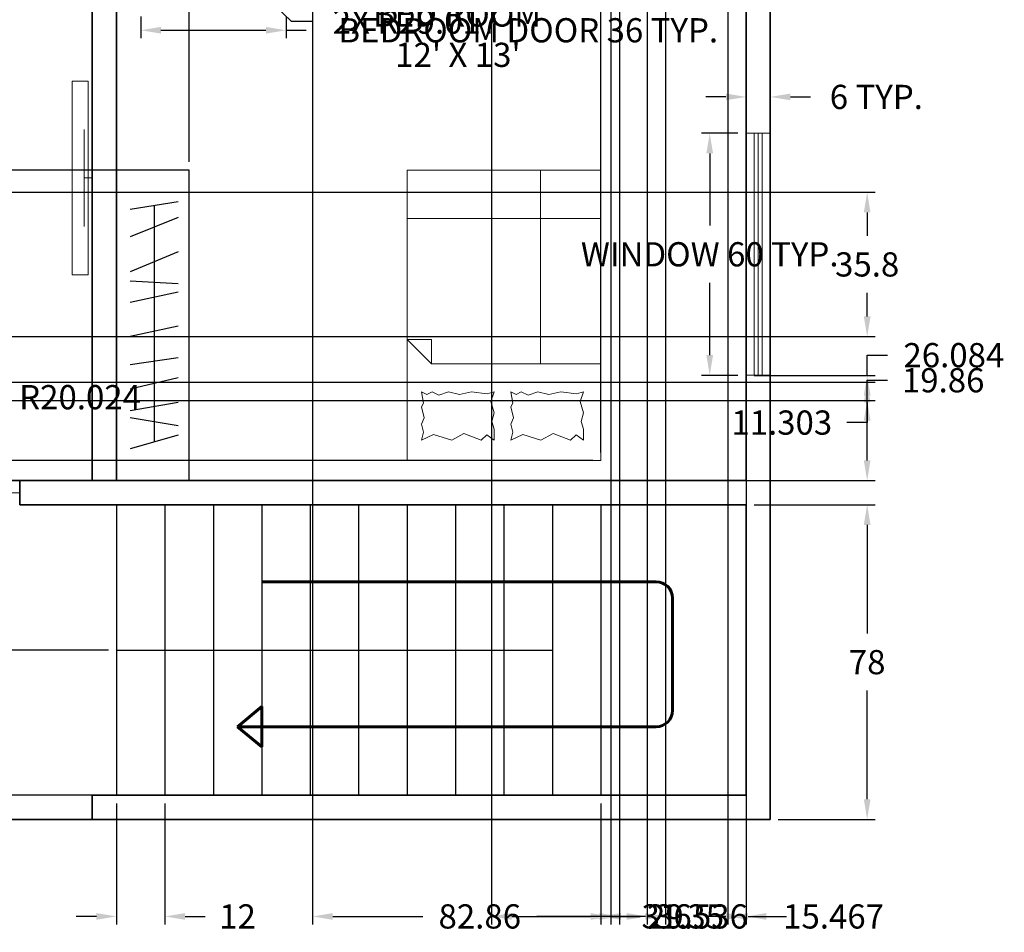
# Model space of a CAD drawing. Units: inches. Extents: x 185 to 668, y 153 to 689.
# Tile 2 of 5: x 417 to 661, y 153 to 380. Entities that reach past the tile are written whole.
import ezdxf

# ---------------------------------------------------------------- set-up
doc = ezdxf.new("R2010")
doc.units = ezdxf.units.IN
doc.header["$MEASUREMENT"] = 0
for name, color, linetype, lineweight in [('A-ANNO-DIMS', 2, 'Continuous', 18), ('A-ANNO-SYMB', 2, 'Continuous', 60), ('A-AREA-IDEN', 7, 'Continuous', 25), ('A-DOOR', 3, 'Continuous', 18), ('A-EQPM', 9, 'Continuous', 18), ('A-FLOR-CASE', 8, 'Continuous', 25), ('A-FLOR-STRS', 7, 'Continuous', 25), ('A-FURN', 8, 'Continuous', 18), ('A-GLAZ', 4, 'Continuous', 18), ('A-WALL', 7, 'Continuous', 35)]:
    doc.layers.add(name, color=color, linetype=linetype, lineweight=lineweight)
doc.styles.get("Standard").update_dxf_attribs({"font": 'arial.ttf'})
doc.dimstyles.get("Standard").update_dxf_attribs({"dimtxt": 6, "dimasz": 5, "dimexe": 2, "dimexo": 2, "dimgap": 4, "dimtad": 0, "dimtih": 1, "dimtoh": 1, "dimdec": 0, "dimzin": 0, "dimdsep": 46, "dimlunit": 3, "dimtxsty": 'Standard', "dimcen": 2, "dimadec": 0, "dimazin": 0, "dimtfac": 1, "dimtdec": 0, "dimtofl": 0, "dimtmove": 0, "dimatfit": 3, "dimfxl": 1, "dimtolj": 1, "dimtzin": 0, "dimarcsym": 0})

# ---------------------------------------------------------------- blocks, each defined once
blk = doc.blocks.new('BED-DOUBLE-48X72')
for p, q in [((0, 72), (48, 72)), ((0, 0), (0, 72)), ((0, 72), (48, 72)), ((0, 0), (0, 72)), ((48, 72), (48, 0)), ((3.52, 66.93), (6.5, 65.56)), ((4.06, 65), (3.52, 66.93)), ((3.52, 66.93), (6.5, 65.56)), ((4.06, 65), (3.52, 66.93)), ((6.5, 65.56), (11.02, 66.93)), ((6.5, 65.56), (11.02, 66.93)), ((11.02, 66.93), (14.02, 65.28)), ((11.02, 66.93), (14.02, 65.28)), ((14.02, 65.28), (18.3, 66.93)), ((14.02, 65.28), (18.3, 66.93)), ((18.3, 66.93), (19.74, 65.6)), ((18.3, 66.93), (19.74, 65.6)), ((19.74, 65.6), (21.52, 66.93)), ((19.74, 65.6), (21.52, 66.93)), ((21.52, 66.93), (21.52, 64.24)), ((21.52, 66.93), (21.52, 64.24)), ((25.65, 66.93), (28.63, 65.56)), ((26.19, 65), (25.65, 66.93)), ((25.65, 66.93), (28.63, 65.56)), ((26.19, 65), (25.65, 66.93)), ((28.63, 65.56), (33.15, 66.93)), ((28.63, 65.56), (33.15, 66.93)), ((33.15, 66.93), (36.15, 65.28)), ((33.15, 66.93), (36.15, 65.28)), ((36.15, 65.28), (40.43, 66.93)), ((36.15, 65.28), (40.43, 66.93)), ((40.43, 66.93), (41.87, 65.6)), ((40.43, 66.93), (41.87, 65.6)), ((41.87, 65.6), (43.65, 66.93)), ((41.87, 65.6), (43.65, 66.93)), ((43.65, 66.93), (43.65, 64.24)), ((43.65, 66.93), (43.65, 64.24)), ((3.52, 63), (4.06, 65)), ((3.52, 63), (4.06, 65)), ((21.52, 64.24), (20.98, 62.32)), ((21.52, 64.24), (20.98, 62.32)), ((25.65, 63), (26.19, 65)), ((25.65, 63), (26.19, 65)), ((43.65, 64.24), (43.11, 62.32)), ((43.65, 64.24), (43.11, 62.32)), ((4.22, 61.4), (3.52, 63)), ((4.22, 61.4), (3.52, 63)), ((3.52, 58.72), (4.22, 61.4)), ((3.52, 58.72), (4.22, 61.4)), ((20.98, 62.32), (21.52, 60.2)), ((20.98, 62.32), (21.52, 60.2)), ((26.35, 61.4), (25.65, 63)), ((26.35, 61.4), (25.65, 63)), ((25.65, 58.72), (26.35, 61.4)), ((25.65, 58.72), (26.35, 61.4)), ((43.11, 62.32), (43.65, 60.2)), ((43.11, 62.32), (43.65, 60.2)), ((4.06, 57.76), (3.52, 58.72)), ((4.06, 57.76), (3.52, 58.72)), ((21.52, 60.2), (20.7, 57.36)), ((21.52, 60.2), (20.7, 57.36)), ((26.19, 57.76), (25.65, 58.72)), ((26.19, 57.76), (25.65, 58.72)), ((43.65, 60.2), (42.83, 57.36)), ((43.65, 60.2), (42.83, 57.36)), ((3.52, 54.93), (4.06, 57.76)), ((3.52, 54.93), (4.06, 57.76)), ((20.7, 57.36), (21.52, 54.93)), ((20.7, 57.36), (21.52, 54.93)), ((25.65, 54.93), (26.19, 57.76)), ((25.65, 54.93), (26.19, 57.76)), ((42.83, 57.36), (43.65, 54.93)), ((42.83, 57.36), (43.65, 54.93)), ((4.9, 55.65), (3.52, 54.93)), ((4.9, 55.65), (3.52, 54.93)), ((6.14, 54.93), (4.9, 55.65)), ((6.14, 54.93), (4.9, 55.65)), ((7.86, 55.8), (6.14, 54.93)), ((7.86, 55.8), (6.14, 54.93)), ((10.22, 54.93), (7.86, 55.8)), ((10.22, 54.93), (7.86, 55.8)), ((12.98, 55.61), (10.22, 54.93)), ((12.98, 55.61), (10.22, 54.93)), ((15.94, 54.93), (12.98, 55.61)), ((15.94, 54.93), (12.98, 55.61)), ((19.78, 55.49), (15.94, 54.93)), ((19.78, 55.49), (15.94, 54.93)), ((21.52, 54.93), (19.78, 55.49)), ((21.52, 54.93), (19.78, 55.49)), ((27.03, 55.65), (25.65, 54.93)), ((27.03, 55.65), (25.65, 54.93)), ((28.27, 54.93), (27.03, 55.65)), ((28.27, 54.93), (27.03, 55.65)), ((29.99, 55.8), (28.27, 54.93)), ((29.99, 55.8), (28.27, 54.93)), ((32.35, 54.93), (29.99, 55.8)), ((32.35, 54.93), (29.99, 55.8)), ((35.11, 55.61), (32.35, 54.93)), ((35.11, 55.61), (32.35, 54.93)), ((38.07, 54.93), (35.11, 55.61)), ((38.07, 54.93), (35.11, 55.61)), ((41.91, 55.49), (38.07, 54.93)), ((41.91, 55.49), (38.07, 54.93)), ((43.65, 54.93), (41.91, 55.49)), ((43.65, 54.93), (41.91, 55.49)), ((0, 42), (6, 48)), ((0, 42), (6, 48)), ((6, 48), (48, 48)), ((6, 48), (6, 42)), ((6, 48), (48, 48)), ((6, 48), (6, 42)), ((33, 48), (33, 0)), ((33, 48), (33, 0)), ((0, 42), (0, 0)), ((0, 42), (6, 42)), ((0, 42), (0, 0)), ((0, 42), (6, 42)), ((48, 12), (0, 12)), ((48, 12), (0, 12)), ((48, 0), (0, 0)), ((48, 0), (0, 0))]:
    blk.add_line(p, q)
blk = doc.blocks.new('WINDOW-60')
for p, q in [((2, 60), (0, 60)), ((2, 60), (2, 0)), ((4, 60), (2, 60)), ((3, 0), (3, 60)), ((4, 0), (4, 60)), ((4, 60), (6, 60)), ((6, 0), (0, 0)), ((2, 0), (0, 0)), ((2, 0), (4, 0)), ((4, 0), (6, 0))]:
    blk.add_line(p, q)
blk = doc.blocks.new('*D9')
at = {"layer": 'A-ANNO-DIMS', "color": 0, "lineweight": -2, "transparency": 16777216}
for p, q in [((595.04, 351.46), (586.04, 351.46)), ((588.04, 346.46), (588.04, 328.57)), ((588.04, 296.46), (588.04, 314.36)), ((595.04, 291.46), (586.04, 291.46))]:
    blk.add_line(p, q, dxfattribs=at)
at = {"layer": 'A-ANNO-DIMS', "color": 0, "transparency": 16777216}
for points in [[(587.21, 346.46), (588.87, 346.46), (588.04, 351.46)], [(587.21, 296.46), (588.87, 296.46), (588.04, 291.46)]]:
    blk.add_solid(points, dxfattribs=at)
at = {"layer": 'Defpoints', "color": 0, "transparency": 16777216}
for p in [(588.04, 351.46), (597.04, 351.46), (597.04, 291.46)]:
    blk.add_point(p, dxfattribs=at)
at = {"layer": 'A-ANNO-DIMS', "color": 0, "transparency": 16777216, "insert": (588.04, 321.46), "char_height": 6, "attachment_point": 5}
blk.add_mtext('\\A1;WINDOW 60 TYP.', dxfattribs=at)
blk = doc.blocks.new('*D10')
at = {"layer": 'A-ANNO-DIMS', "color": 0, "lineweight": -2, "transparency": 16777216}
for p, q in [((597.04, 353.46), (597.04, 362.46)), ((603.04, 353.46), (603.04, 362.46)), ((592.04, 360.46), (587.04, 360.46)), ((608.04, 360.46), (613.04, 360.46))]:
    blk.add_line(p, q, dxfattribs=at)
at = {"layer": 'A-ANNO-DIMS', "color": 0, "transparency": 16777216}
for points in [[(592.04, 361.3), (592.04, 359.63), (597.04, 360.46)], [(608.04, 361.3), (608.04, 359.63), (603.04, 360.46)]]:
    blk.add_solid(points, dxfattribs=at)
at = {"layer": 'Defpoints', "color": 0, "transparency": 16777216}
for p in [(603.04, 360.46), (597.04, 351.46), (603.04, 351.46)]:
    blk.add_point(p, dxfattribs=at)
at = {"layer": 'A-ANNO-DIMS', "color": 0, "transparency": 16777216, "insert": (629.33, 360.46), "char_height": 6, "attachment_point": 5}
blk.add_mtext('\\A1;6 TYP.', dxfattribs=at)
blk = doc.blocks.new('*D21')
at = {"layer": 'A-ANNO-DIMS', "color": 0, "lineweight": -2, "transparency": 16777216}
for p, q in [((447.04, 380.38), (447.04, 374.98)), ((483.04, 380.38), (483.04, 374.98)), ((452.04, 376.98), (478.04, 376.98)), ((483.04, 376.98), (488.04, 376.98))]:
    blk.add_line(p, q, dxfattribs=at)
at = {"layer": 'A-ANNO-DIMS', "color": 0, "transparency": 16777216}
for points in [[(452.04, 377.81), (452.04, 376.15), (447.04, 376.98)], [(478.04, 377.81), (478.04, 376.15), (483.04, 376.98)]]:
    blk.add_solid(points, dxfattribs=at)
at = {"layer": 'Defpoints', "color": 0, "transparency": 16777216}
for p in [(447.04, 382.38), (483.04, 382.38), (483.04, 376.98)]:
    blk.add_point(p, dxfattribs=at)
at = {"layer": 'A-ANNO-DIMS', "color": 0, "transparency": 16777216, "insert": (543.07, 376.98), "char_height": 6, "attachment_point": 5}
blk.add_mtext('\\A1;BEDROOM DOOR 36 TYP.', dxfattribs=at)
blk = doc.blocks.new('*D27')
at = {"layer": 'A-ANNO-DIMS', "color": 0, "lineweight": -2, "transparency": 16777216}
for p, q in [((599.04, 259.38), (629.06, 259.38)), ((627.06, 254.38), (627.06, 227.44)), ((627.06, 186.38), (627.06, 213.32)), ((605.04, 181.38), (629.06, 181.38))]:
    blk.add_line(p, q, dxfattribs=at)
at = {"layer": 'A-ANNO-DIMS', "color": 0, "transparency": 16777216}
for points in [[(626.23, 254.38), (627.89, 254.38), (627.06, 259.38)], [(626.23, 186.38), (627.89, 186.38), (627.06, 181.38)]]:
    blk.add_solid(points, dxfattribs=at)
at = {"layer": 'Defpoints', "color": 0, "transparency": 16777216}
for p in [(597.04, 259.38), (627.06, 259.38), (603.04, 181.38)]:
    blk.add_point(p, dxfattribs=at)
at = {"layer": 'A-ANNO-DIMS', "color": 0, "transparency": 16777216, "insert": (627.06, 220.38), "char_height": 6, "attachment_point": 5}
blk.add_mtext('\\A1;78', dxfattribs=at)
blk = doc.blocks.new('*D28')
at = {"layer": 'A-ANNO-DIMS', "color": 0, "lineweight": -2, "transparency": 16777216}
for p, q in [((627.06, 285.24), (627.06, 290.24)), ((627.06, 290.24), (632.06, 290.24)), ((251.04, 285.24), (629.06, 285.24)), ((627.06, 270.38), (627.06, 280.24)), ((251.04, 265.38), (629.06, 265.38))]:
    blk.add_line(p, q, dxfattribs=at)
at = {"layer": 'A-ANNO-DIMS', "color": 0, "transparency": 16777216}
for points in [[(626.23, 280.24), (627.89, 280.24), (627.06, 285.24)], [(626.23, 270.38), (627.89, 270.38), (627.06, 265.38)]]:
    blk.add_solid(points, dxfattribs=at)
at = {"layer": 'Defpoints', "color": 0, "transparency": 16777216}
for p in [(249.04, 285.24), (627.06, 285.24), (249.04, 265.38)]:
    blk.add_point(p, dxfattribs=at)
at = {"layer": 'A-ANNO-DIMS', "color": 0, "transparency": 16777216, "insert": (645.9, 290.24), "char_height": 6, "attachment_point": 5}
blk.add_mtext('\\A1;19.86', dxfattribs=at)
blk = doc.blocks.new('*D29')
at = {"layer": 'A-ANNO-DIMS', "color": 0, "lineweight": -2, "transparency": 16777216}
for p, q in [((627.06, 291.46), (627.06, 296.46)), ((627.06, 296.46), (632.06, 296.46)), ((599.04, 291.46), (629.06, 291.46)), ((627.06, 270.38), (627.06, 286.46)), ((599.04, 265.38), (629.06, 265.38))]:
    blk.add_line(p, q, dxfattribs=at)
at = {"layer": 'A-ANNO-DIMS', "color": 0, "transparency": 16777216}
for points in [[(626.23, 286.46), (627.89, 286.46), (627.06, 291.46)], [(626.23, 270.38), (627.89, 270.38), (627.06, 265.38)]]:
    blk.add_solid(points, dxfattribs=at)
at = {"layer": 'Defpoints', "color": 0, "transparency": 16777216}
for p in [(597.04, 291.46), (627.06, 291.46), (597.04, 265.38)]:
    blk.add_point(p, dxfattribs=at)
at = {"layer": 'A-ANNO-DIMS', "color": 0, "transparency": 16777216, "insert": (648.55, 296.46), "char_height": 6, "attachment_point": 5}
blk.add_mtext('\\A1;26.084', dxfattribs=at)
blk = doc.blocks.new('*D33')
at = {"layer": 'A-ANNO-DIMS', "color": 0, "lineweight": -2, "transparency": 16777216}
for p, q in [((565.69, 653.38), (565.69, 155.36)), ((597.04, 653.38), (597.04, 155.36)), ((560.69, 157.36), (555.69, 157.36)), ((602.04, 157.36), (607.04, 157.36))]:
    blk.add_line(p, q, dxfattribs=at)
at = {"layer": 'A-ANNO-DIMS', "color": 0, "transparency": 16777216}
for points in [[(560.69, 158.19), (560.69, 156.53), (565.69, 157.36)], [(602.04, 158.19), (602.04, 156.53), (597.04, 157.36)]]:
    blk.add_solid(points, dxfattribs=at)
at = {"layer": 'Defpoints', "color": 0, "transparency": 16777216}
for p in [(565.69, 655.38), (597.04, 655.38), (597.04, 157.36)]:
    blk.add_point(p, dxfattribs=at)
at = {"layer": 'A-ANNO-DIMS', "color": 0, "transparency": 16777216, "insert": (581.37, 157.36), "char_height": 6, "attachment_point": 5}
blk.add_mtext('\\A1;31.35', dxfattribs=at)
blk = doc.blocks.new('*D39')
at = {"layer": 'A-ANNO-DIMS', "color": 0, "lineweight": -2, "transparency": 16777216}
for p, q in [((441.04, 185.38), (441.04, 155.36)), ((453.04, 185.38), (453.04, 155.36)), ((436.04, 157.36), (431.04, 157.36)), ((458.04, 157.36), (463.04, 157.36))]:
    blk.add_line(p, q, dxfattribs=at)
at = {"layer": 'A-ANNO-DIMS', "color": 0, "transparency": 16777216}
for points in [[(436.04, 158.19), (436.04, 156.53), (441.04, 157.36)], [(458.04, 158.19), (458.04, 156.53), (453.04, 157.36)]]:
    blk.add_solid(points, dxfattribs=at)
at = {"layer": 'Defpoints', "color": 0, "transparency": 16777216}
for p in [(441.04, 187.38), (453.04, 187.38), (453.04, 157.36)]:
    blk.add_point(p, dxfattribs=at)
at = {"layer": 'A-ANNO-DIMS', "color": 0, "transparency": 16777216, "insert": (471.03, 157.36), "char_height": 6, "attachment_point": 5}
blk.add_mtext('\\A1;12', dxfattribs=at)
blk = doc.blocks.new('*D43')
at = {"layer": 'A-ANNO-DIMS', "color": 0, "lineweight": -2, "transparency": 16777216}
for p, q in [((489.63, 629.38), (489.63, 155.36)), ((572.5, 629.38), (572.5, 155.36)), ((494.63, 157.36), (516.94, 157.36)), ((567.5, 157.36), (545.19, 157.36))]:
    blk.add_line(p, q, dxfattribs=at)
at = {"layer": 'A-ANNO-DIMS', "color": 0, "transparency": 16777216}
for points in [[(494.63, 158.19), (494.63, 156.53), (489.63, 157.36)], [(567.5, 158.19), (567.5, 156.53), (572.5, 157.36)]]:
    blk.add_solid(points, dxfattribs=at)
at = {"layer": 'Defpoints', "color": 0, "transparency": 16777216}
for p in [(489.63, 631.38), (572.5, 631.38), (572.5, 157.36)]:
    blk.add_point(p, dxfattribs=at)
at = {"layer": 'A-ANNO-DIMS', "color": 0, "transparency": 16777216, "insert": (531.06, 157.36), "char_height": 6, "attachment_point": 5}
blk.add_mtext('\\A1;82.86', dxfattribs=at)
blk = doc.blocks.new('*D52')
at = {"layer": 'A-ANNO-DIMS', "color": 0, "lineweight": -2, "transparency": 16777216}
for p, q in [((441.04, 344.34), (441.04, 687.4)), ((459.04, 344.34), (459.04, 687.4)), ((436.04, 685.4), (431.04, 685.4)), ((464.04, 685.4), (469.04, 685.4))]:
    blk.add_line(p, q, dxfattribs=at)
at = {"layer": 'A-ANNO-DIMS', "color": 0, "transparency": 16777216}
for points in [[(436.04, 686.23), (436.04, 684.56), (441.04, 685.4)], [(464.04, 686.23), (464.04, 684.56), (459.04, 685.4)]]:
    blk.add_solid(points, dxfattribs=at)
at = {"layer": 'Defpoints', "color": 0, "transparency": 16777216}
for p in [(459.04, 685.4), (441.04, 342.34), (459.04, 342.34)]:
    blk.add_point(p, dxfattribs=at)
at = {"layer": 'A-ANNO-DIMS', "color": 0, "transparency": 16777216, "insert": (450.04, 685.4), "char_height": 6, "attachment_point": 5}
blk.add_mtext('\\A1;18', dxfattribs=at)
blk = doc.blocks.new('*D53')
at = {"layer": 'A-ANNO-DIMS', "color": 0, "lineweight": -2, "transparency": 16777216}
for p, q in [((457.04, 342.34), (217.02, 342.34)), ((219.02, 337.34), (219.02, 310.92)), ((219.02, 270.38), (219.02, 296.79)), ((457.04, 265.38), (217.02, 265.38))]:
    blk.add_line(p, q, dxfattribs=at)
at = {"layer": 'A-ANNO-DIMS', "color": 0, "transparency": 16777216}
for points in [[(218.19, 337.34), (219.86, 337.34), (219.02, 342.34)], [(218.19, 270.38), (219.86, 270.38), (219.02, 265.38)]]:
    blk.add_solid(points, dxfattribs=at)
at = {"layer": 'Defpoints', "color": 0, "transparency": 16777216}
for p in [(219.02, 342.34), (459.04, 342.34), (459.04, 265.38)]:
    blk.add_point(p, dxfattribs=at)
at = {"layer": 'A-ANNO-DIMS', "color": 0, "transparency": 16777216, "insert": (219.02, 303.86), "char_height": 6, "attachment_point": 5}
blk.add_mtext('\\A1;76.96', dxfattribs=at)
blk = doc.blocks.new('*D55')
at = {"layer": 'A-ANNO-DIMS', "color": 0, "lineweight": -2, "transparency": 16777216}
for p, q in [((313.16, 336.85), (629.06, 336.85)), ((627.06, 331.85), (627.06, 326.02)), ((627.06, 306.05), (627.06, 311.89)), ((313.16, 301.05), (629.06, 301.05))]:
    blk.add_line(p, q, dxfattribs=at)
at = {"layer": 'A-ANNO-DIMS', "color": 0, "transparency": 16777216}
for points in [[(626.23, 331.85), (627.89, 331.85), (627.06, 336.85)], [(626.23, 306.05), (627.89, 306.05), (627.06, 301.05)]]:
    blk.add_solid(points, dxfattribs=at)
at = {"layer": 'Defpoints', "color": 0, "transparency": 16777216}
for p in [(311.16, 336.85), (627.06, 336.85), (311.16, 301.05)]:
    blk.add_point(p, dxfattribs=at)
at = {"layer": 'A-ANNO-DIMS', "color": 0, "transparency": 16777216, "insert": (627.06, 318.95), "char_height": 6, "attachment_point": 5}
blk.add_mtext('\\A1;35.8', dxfattribs=at)
blk = doc.blocks.new('*D59')
at = {"layer": 'A-ANNO-DIMS', "color": 0, "lineweight": -2, "transparency": 16777216}
for p, q in [((627.06, 306.05), (627.06, 311.05)), ((289.14, 301.05), (629.06, 301.05)), ((297.85, 289.75), (629.06, 289.75)), ((627.06, 284.75), (627.06, 279.75)), ((627.06, 279.75), (622.06, 279.75))]:
    blk.add_line(p, q, dxfattribs=at)
at = {"layer": 'A-ANNO-DIMS', "color": 0, "transparency": 16777216}
for points in [[(626.23, 306.05), (627.89, 306.05), (627.06, 301.05)], [(626.23, 284.75), (627.89, 284.75), (627.06, 289.75)]]:
    blk.add_solid(points, dxfattribs=at)
at = {"layer": 'Defpoints', "color": 0, "transparency": 16777216}
for p in [(287.14, 301.05), (295.85, 289.75), (627.06, 289.75)]:
    blk.add_point(p, dxfattribs=at)
at = {"layer": 'A-ANNO-DIMS', "color": 0, "transparency": 16777216, "insert": (605.89, 279.75), "char_height": 6, "attachment_point": 5}
blk.add_mtext('\\A1;11.303', dxfattribs=at)
blk = doc.blocks.new('*D60')
at = {"layer": 'A-ANNO-DIMS', "color": 0, "lineweight": -2, "transparency": 16777216}
for p, q in [((439.04, 223.38), (217.02, 223.38)), ((219.02, 218.38), (219.02, 212.44)), ((219.02, 192.38), (219.02, 198.31)), ((439.04, 187.38), (217.02, 187.38))]:
    blk.add_line(p, q, dxfattribs=at)
at = {"layer": 'A-ANNO-DIMS', "color": 0, "transparency": 16777216}
for points in [[(218.19, 218.38), (219.86, 218.38), (219.02, 223.38)], [(218.19, 192.38), (219.86, 192.38), (219.02, 187.38)]]:
    blk.add_solid(points, dxfattribs=at)
at = {"layer": 'Defpoints', "color": 0, "transparency": 16777216}
for p in [(219.02, 223.38), (441.04, 223.38), (441.04, 187.38)]:
    blk.add_point(p, dxfattribs=at)
at = {"layer": 'A-ANNO-DIMS', "color": 0, "transparency": 16777216, "insert": (219.02, 205.38), "char_height": 6, "attachment_point": 5}
blk.add_mtext('\\A1;36', dxfattribs=at)
blk = doc.blocks.new('*D61')
at = {"layer": 'A-ANNO-DIMS', "color": 0, "lineweight": -2, "transparency": 16777216}
for p, q in [((561.04, 185.38), (561.04, 155.36)), ((597.04, 185.38), (597.04, 155.36)), ((566.04, 157.36), (570.75, 157.36)), ((592.04, 157.36), (587.33, 157.36))]:
    blk.add_line(p, q, dxfattribs=at)
at = {"layer": 'A-ANNO-DIMS', "color": 0, "transparency": 16777216}
for points in [[(566.04, 158.19), (566.04, 156.53), (561.04, 157.36)], [(592.04, 158.19), (592.04, 156.53), (597.04, 157.36)]]:
    blk.add_solid(points, dxfattribs=at)
at = {"layer": 'Defpoints', "color": 0, "transparency": 16777216}
for p in [(561.04, 187.38), (597.04, 187.38), (597.04, 157.36)]:
    blk.add_point(p, dxfattribs=at)
at = {"layer": 'A-ANNO-DIMS', "color": 0, "transparency": 16777216, "insert": (579.04, 157.36), "char_height": 6, "attachment_point": 5}
blk.add_mtext('\\A1;36', dxfattribs=at)
blk = doc.blocks.new('*D62')
at = {"layer": 'A-ANNO-DIMS', "color": 0, "lineweight": -2, "transparency": 16777216}
for p, q in [((533.97, 632.47), (533.97, 155.36)), ((563.51, 632.47), (563.51, 155.36)), ((538.97, 157.36), (558.51, 157.36)), ((563.51, 157.36), (568.51, 157.36))]:
    blk.add_line(p, q, dxfattribs=at)
at = {"layer": 'A-ANNO-DIMS', "color": 0, "transparency": 16777216}
for points in [[(538.97, 158.19), (538.97, 156.53), (533.97, 157.36)], [(558.51, 158.19), (558.51, 156.53), (563.51, 157.36)]]:
    blk.add_solid(points, dxfattribs=at)
at = {"layer": 'Defpoints', "color": 0, "transparency": 16777216}
for p in [(533.97, 634.47), (563.51, 634.47), (563.51, 157.36)]:
    blk.add_point(p, dxfattribs=at)
at = {"layer": 'A-ANNO-DIMS', "color": 0, "transparency": 16777216, "insert": (585.01, 157.36), "char_height": 6, "attachment_point": 5}
blk.add_mtext('\\A1;29.536', dxfattribs=at)
blk = doc.blocks.new('*D65')
at = {"layer": 'A-ANNO-DIMS', "color": 0, "lineweight": -2, "transparency": 16777216}
for p, q in [((577.09, 545.77), (577.09, 155.36)), ((592.55, 545.77), (592.55, 155.36)), ((572.09, 157.36), (567.09, 157.36)), ((597.55, 157.36), (602.55, 157.36))]:
    blk.add_line(p, q, dxfattribs=at)
at = {"layer": 'A-ANNO-DIMS', "color": 0, "transparency": 16777216}
for points in [[(572.09, 158.19), (572.09, 156.53), (577.09, 157.36)], [(597.55, 158.19), (597.55, 156.53), (592.55, 157.36)]]:
    blk.add_solid(points, dxfattribs=at)
at = {"layer": 'Defpoints', "color": 0, "transparency": 16777216}
for p in [(577.09, 547.77), (592.55, 547.77), (592.55, 157.36)]:
    blk.add_point(p, dxfattribs=at)
at = {"layer": 'A-ANNO-DIMS', "color": 0, "transparency": 16777216, "insert": (618.73, 157.36), "char_height": 6, "attachment_point": 5}
blk.add_mtext('\\A1;15.467', dxfattribs=at)
blk = doc.blocks.new('*D74')
at = {"layer": 'A-ANNO-DIMS', "color": 0, "lineweight": -2, "transparency": 16777216}
for p, q in [((561.08, 272.34), (561.08, 687.4)), ((597.04, 267.38), (597.04, 687.4)), ((556.08, 685.4), (551.08, 685.4)), ((602.04, 685.4), (607.04, 685.4))]:
    blk.add_line(p, q, dxfattribs=at)
at = {"layer": 'A-ANNO-DIMS', "color": 0, "transparency": 16777216}
for points in [[(556.08, 686.23), (556.08, 684.56), (561.08, 685.4)], [(602.04, 686.23), (602.04, 684.56), (597.04, 685.4)]]:
    blk.add_solid(points, dxfattribs=at)
at = {"layer": 'Defpoints', "color": 0, "transparency": 16777216}
for p in [(597.04, 685.4), (561.08, 270.34), (597.04, 265.38)]:
    blk.add_point(p, dxfattribs=at)
at = {"layer": 'A-ANNO-DIMS', "color": 0, "transparency": 16777216, "insert": (579.06, 685.4), "char_height": 6, "attachment_point": 5}
blk.add_mtext('\\A1;35.96', dxfattribs=at)
blk = doc.blocks.new('*D75')
at = {"layer": 'A-ANNO-DIMS', "color": 0, "lineweight": -2, "transparency": 16777216}
for p, q in [((219.02, 275.34), (219.02, 280.34)), ((559.08, 270.34), (217.02, 270.34)), ((595.04, 265.38), (217.02, 265.38)), ((219.02, 260.38), (219.02, 255.38)), ((219.02, 255.38), (214.02, 255.38))]:
    blk.add_line(p, q, dxfattribs=at)
at = {"layer": 'A-ANNO-DIMS', "color": 0, "transparency": 16777216}
for points in [[(218.19, 275.34), (219.86, 275.34), (219.02, 270.34)], [(218.19, 260.38), (219.86, 260.38), (219.02, 265.38)]]:
    blk.add_solid(points, dxfattribs=at)
at = {"layer": 'Defpoints', "color": 0, "transparency": 16777216}
for p in [(561.08, 270.34), (219.02, 265.38), (597.04, 265.38)]:
    blk.add_point(p, dxfattribs=at)
at = {"layer": 'A-ANNO-DIMS', "color": 0, "transparency": 16777216, "insert": (199.78, 255.38), "char_height": 6, "attachment_point": 5}
blk.add_mtext('\\A1;4.957', dxfattribs=at)
blk = doc.blocks.new('*D76')
at = {"layer": 'A-ANNO-DIMS', "color": 0, "lineweight": -2, "transparency": 16777216}
for p, q in [((395.66, 286.05), (390.71, 281.08)), ((400.66, 286.05), (395.66, 286.05)), ((373.04, 261.36), (373.04, 265.36)), ((371.04, 263.36), (375.04, 263.36))]:
    blk.add_line(p, q, dxfattribs=at)
at = {"layer": 'A-ANNO-DIMS', "color": 0, "transparency": 16777216}
blk.add_solid([(390.12, 281.67), (391.3, 280.49), (387.18, 277.54)], dxfattribs=at)
at = {"layer": 'Defpoints', "color": 0, "transparency": 16777216}
for p in [(387.18, 277.54), (373.04, 263.36)]:
    blk.add_point(p, dxfattribs=at)
at = {"layer": 'A-ANNO-DIMS', "color": 0, "transparency": 16777216, "insert": (426.47, 286.05), "char_height": 6, "attachment_point": 5}
blk.add_mtext('\\A1;2X R20.024', dxfattribs=at)
blk = doc.blocks.new('*D77')
at = {"layer": 'A-ANNO-DIMS', "color": 0, "lineweight": -2, "transparency": 16777216}
for p, q in [((451.04, 409.4), (451.04, 413.4)), ((449.04, 411.4), (453.04, 411.4)), ((484.42, 379.13), (475.5, 387.75)), ((489.42, 379.13), (484.42, 379.13))]:
    blk.add_line(p, q, dxfattribs=at)
at = {"layer": 'A-ANNO-DIMS', "color": 0, "transparency": 16777216}
blk.add_solid([(476.08, 388.35), (474.92, 387.15), (471.9, 391.23)], dxfattribs=at)
at = {"layer": 'Defpoints', "color": 0, "transparency": 16777216}
for p in [(451.04, 411.4), (471.9, 391.23)]:
    blk.add_point(p, dxfattribs=at)
at = {"layer": 'A-ANNO-DIMS', "color": 0, "transparency": 16777216, "insert": (515.24, 379.13), "char_height": 6, "attachment_point": 5}
blk.add_mtext('\\A1;2X R29.017', dxfattribs=at)

msp = doc.modelspace()

# ---------------------------------------------------------------- linework, layer by layer
at = {"layer": 'A-ANNO-SYMB'}
for p, q in [((477.041, 240.2891), (574.8028, 240.2891)), ((578.8028, 236.2891), (578.8028, 208.3708)), ((477.041, 209.3708), (471.041, 204.3708)), ((477.041, 204.3708), (477.041, 209.3708)), ((477.041, 204.3708), (471.041, 204.3708)), ((477.041, 199.3708), (471.041, 204.3708)), ((574.8028, 204.3708), (477.041, 204.3708)), ((477.041, 204.3708), (477.041, 199.3708))]:
    msp.add_line(p, q, dxfattribs=at)
for centre, start, end in [((574.8028, 236.2891), 0, 90), ((574.8028, 208.3708), 270, 0)]:
    msp.add_arc(centre, 4, start, end, dxfattribs=at)
at = {"layer": 'A-DOOR'}
msp.add_line((417.041, 262.3789), (414.041, 262.3789), dxfattribs=at)
at = {"layer": 'A-EQPM'}
for p, q in [((430.041, 316.3789), (430.041, 364.3789)), ((430.041, 364.3789), (434.041, 364.3789)), ((434.041, 364.3789), (434.041, 340.3789)), ((433.041, 340.3789), (433.041, 352.3789)), ((434.041, 340.3789), (433.041, 340.3789)), ((433.041, 340.3789), (433.041, 328.3789)), ((435.041, 340.3789), (434.041, 340.3789)), ((434.041, 340.3789), (434.041, 316.3789)), ((434.041, 316.3789), (430.041, 316.3789))]:
    msp.add_line(p, q, dxfattribs=at)
at = {"layer": 'A-FLOR-CASE'}
for p, q in [((459.041, 342.3357), (441.041, 342.3357)), ((459.041, 265.3789), (459.041, 342.3357)), ((444.389, 332.6743), (456.3053, 334.5661)), ((450.3472, 333.6202), (450.3472, 274.9403)), ((456.3053, 330.56), (444.389, 325.7453)), ((456.3053, 322.0336), (444.389, 317.1465)), ((444.389, 314.8665), (456.3053, 314.2303)), ((456.3053, 312.0432), (444.389, 309.5316)), ((456.3053, 303.6634), (444.389, 301.079)), ((456.3053, 295.7764), (444.389, 294.0755)), ((456.3053, 290.842), (444.389, 288.0574)), ((456.3053, 284.7672), (444.389, 282.641)), ((444.389, 281.0103), (456.3053, 279.0258)), ((456.3053, 276.6565), (444.389, 273.224)), ((441.041, 265.3789), (459.041, 265.3789))]:
    msp.add_line(p, q, dxfattribs=at)
at = {"layer": 'A-FLOR-STRS'}
for p, q in [((441.041, 259.3789), (441.041, 187.3789)), ((453.041, 259.3789), (453.041, 187.3789)), ((465.041, 259.3789), (465.041, 187.3789)), ((477.041, 259.3789), (477.041, 187.3789)), ((489.041, 259.3789), (489.041, 187.3789)), ((501.041, 259.3789), (501.041, 187.3789)), ((513.041, 259.3789), (513.041, 187.3789)), ((525.041, 259.3789), (525.041, 187.3789)), ((537.041, 259.3789), (537.041, 187.3789)), ((549.041, 259.3789), (549.041, 187.3789)), ((561.041, 259.3789), (561.041, 187.3789)), ((441.041, 223.3789), (549.041, 223.3789))]:
    msp.add_line(p, q, dxfattribs=at)
at = {"layer": 'A-FURN'}
msp.add_line((561.0793, 270.3357), (561.0793, 342.3357), dxfattribs=at)
msp.add_line((561.0793, 270.3357), (561.0793, 342.3357), dxfattribs=at)
at = {"layer": 'A-WALL'}
for p, q in [((603.041, 181.3789), (603.041, 661.3789)), ((435.041, 415.3789), (435.041, 265.3789)), ((441.041, 265.3789), (441.041, 409.3789)), ((597.041, 409.3789), (597.041, 265.3789)), ((435.041, 265.3789), (417.041, 265.3789)), ((417.041, 265.3789), (417.041, 259.3789)), ((597.041, 265.3789), (441.041, 265.3789)), ((435.041, 259.3789), (417.041, 259.3789)), ((597.041, 259.3789), (435.041, 259.3789)), ((597.041, 259.3789), (597.041, 187.3789)), ((435.041, 187.3789), (597.041, 187.3789)), ((435.041, 187.3789), (441.041, 187.3789)), ((435.041, 187.3789), (435.041, 181.3789)), ((243.041, 181.3789), (603.041, 181.3789))]:
    msp.add_line(p, q, dxfattribs=at)

# ---------------------------------------------------------------- block references
at = {"layer": 'A-FURN', "extrusion": (0, 0, -1), "zscale": -1, "rotation": 180}
msp.add_blockref('BED-DOUBLE-48X72', (-513.079, 342.3353), dxfattribs=at)
at = {"layer": 'A-GLAZ'}
msp.add_blockref('WINDOW-60', (597.041, 291.4629), dxfattribs=at)

# ---------------------------------------------------------------- texts
at = {"layer": 'A-AREA-IDEN', "insert": (504.606, 383.8904), "char_height": 6, "attachment_point": 1}
msp.add_mtext_dynamic_manual_height_columns("BED ROOM\\P   12' X 13'", width=69.605686, gutter_width=1, heights=[0], dxfattribs=at)

# ---------------------------------------------------------------- dimensions: what is measured, and where the dimension line sits
at = {"layer": 'A-ANNO-DIMS'}
for base, p1, p2, override, picture, middle in [((459.041, 685.3964), (441.041, 342.3357), (459.041, 342.3357), {"dimdec": 0, "dimlfac": 1, "dimrnd": 0, "dimzin": 0, "dimdsep": 46, "dimlunit": 2}, '*D52', (450.041, 685.3964)), ((597.041, 685.3964), (561.0793, 270.3357), (597.041, 265.3789), {"dimdec": 2, "dimlfac": 1, "dimrnd": 0, "dimzin": 0, "dimdsep": 46, "dimlunit": 2}, '*D74', (579.0601, 685.3964)), ((597.041, 157.3614), (565.6925, 655.3789), (597.041, 655.3789), {"dimdec": 2, "dimlfac": 1, "dimrnd": 0, "dimzin": 0, "dimdsep": 46, "dimlunit": 2}, '*D33', (581.3667, 157.3614)), ((563.5058, 157.3614), (533.9695, 634.4736), (563.5058, 634.4736), {"dimdec": 3, "dimlfac": 1, "dimrnd": 0, "dimzin": 0, "dimdsep": 46, "dimlunit": 2}, '*D62', (585.0092, 157.3614)), ((572.4952, 157.3614), (489.6328, 631.3789), (572.4952, 631.3789), {"dimdec": 2, "dimlfac": 1, "dimrnd": 0, "dimzin": 0, "dimdsep": 46, "dimlunit": 2}, '*D43', (531.064, 157.3614)), ((592.5536, 157.3614), (577.0867, 547.7709), (592.5536, 547.7709), {"dimdec": 3, "dimlfac": 1, "dimrnd": 0, "dimzin": 0, "dimdsep": 46, "dimlunit": 2}, '*D65', (618.7255, 157.3614)), ((453.041, 157.3614), (441.041, 187.3789), (453.041, 187.3789), {"dimdec": 0, "dimlfac": 1, "dimrnd": 0, "dimzin": 0, "dimdsep": 46, "dimlunit": 2}, '*D39', (471.0253, 157.3614)), ((597.041, 157.3614), (561.041, 187.3789), (597.041, 187.3789), {"dimdec": 0, "dimlfac": 1, "dimrnd": 0, "dimzin": 0, "dimdsep": 46, "dimlunit": 2}, '*D61', (579.041, 157.3614))]:
    dim = msp.add_linear_dim(base=base, p1=p1, p2=p2, dimstyle='Standard', override=override, dxfattribs=at)
    dim.commit()
    dim.dimension.update_dxf_attribs({"geometry": picture, "text_midpoint": middle})
for center, mpoint, picture, middle in [((451.041, 411.3956), (471.9036, 391.2284), '*D77', (515.2438, 379.128)), ((373.041, 263.3551), (387.1765, 277.5375), '*D76', (426.4682, 286.0469))]:
    dim = msp.add_radius_dim(center=center, mpoint=mpoint, text='2X <>', dimstyle='Standard', override={"dimdec": 3, "dimlfac": 1, "dimrnd": 0, "dimzin": 0, "dimdsep": 46, "dimlunit": 2}, dxfattribs=at)
    dim.commit()
    dim.dimension.update_dxf_attribs({"geometry": picture, "text_midpoint": middle, "dimtype": 164})
for base, p1, p2, text, picture, middle in [((483.041, 376.9789), (447.041, 382.3789), (483.041, 382.3789), 'BEDROOM DOOR <> TYP.', '*D21', (543.0676, 376.9789)), ((603.041, 360.4628), (597.041, 351.4628), (603.041, 351.4628), '<> TYP.', '*D10', (629.3295, 360.4628))]:
    dim = msp.add_linear_dim(base=base, p1=p1, p2=p2, text=text, dimstyle='Standard', override={"dimdec": 0, "dimlfac": 1, "dimrnd": 0, "dimzin": 0, "dimdsep": 46, "dimlunit": 2}, dxfattribs=at)
    dim.commit()
    dim.dimension.update_dxf_attribs({"geometry": picture, "text_midpoint": middle})
dim = msp.add_linear_dim(base=(588.041, 351.4628), p1=(597.041, 291.4628), p2=(597.041, 351.4628), angle=90, text='WINDOW <> TYP.', dimstyle='Standard', override={"dimdec": 0, "dimlfac": 1, "dimrnd": 0, "dimzin": 0, "dimdsep": 46, "dimlunit": 2}, dxfattribs=at)
dim.commit()
dim.dimension.update_dxf_attribs({"geometry": '*D9', "text_midpoint": (588.041, 321.4628)})
for base, p1, p2, override, picture, middle in [((219.0235, 342.3357), (459.041, 265.3789), (459.041, 342.3357), {"dimdec": 2, "dimlfac": 1, "dimrnd": 0, "dimzin": 0, "dimdsep": 46, "dimlunit": 2}, '*D53', (219.0235, 303.8573)), ((627.0585, 336.854), (311.1562, 301.0535), (311.1562, 336.854), {"dimdec": 1, "dimlfac": 1, "dimrnd": 0, "dimzin": 0, "dimdsep": 46, "dimlunit": 2}, '*D55', (627.0585, 318.9537)), ((627.0585, 289.7509), (287.1365, 301.0535), (295.8541, 289.7509), {"dimdec": 3, "dimlfac": 1, "dimrnd": 0, "dimzin": 0, "dimdsep": 46, "dimlunit": 2}, '*D59', (605.8866, 279.7509)), ((627.0585, 291.4628), (597.041, 265.3789), (597.041, 291.4628), {"dimdec": 3, "dimlfac": 1, "dimrnd": 0, "dimzin": 0, "dimdsep": 46, "dimlunit": 2}, '*D29', (648.5516, 296.4628)), ((627.0585, 285.2389), (249.041, 265.3789), (249.041, 285.2389), {"dimdec": 2, "dimlfac": 1, "dimrnd": 0, "dimzin": 0, "dimdsep": 46, "dimlunit": 2}, '*D28', (645.8975, 290.2389)), ((219.0235, 265.3789), (561.0793, 270.3357), (597.041, 265.3789), {"dimdec": 3, "dimlfac": 1, "dimrnd": 0, "dimzin": 0, "dimdsep": 46, "dimlunit": 2}, '*D75', (199.7793, 255.3789)), ((627.0585, 259.3789), (603.041, 181.3789), (597.041, 259.3789), {"dimdec": 0, "dimlfac": 1, "dimrnd": 0, "dimzin": 0, "dimdsep": 46, "dimlunit": 2}, '*D27', (627.0585, 220.3789)), ((219.0235, 223.3789), (441.041, 187.3789), (441.041, 223.3789), {"dimdec": 0, "dimlfac": 1, "dimrnd": 0, "dimzin": 0, "dimdsep": 46, "dimlunit": 2}, '*D60', (219.0235, 205.3789))]:
    dim = msp.add_linear_dim(base=base, p1=p1, p2=p2, angle=90, dimstyle='Standard', override=override, dxfattribs=at)
    dim.commit()
    dim.dimension.update_dxf_attribs({"geometry": picture, "text_midpoint": middle})

doc.saveas('drawing.dxf')
